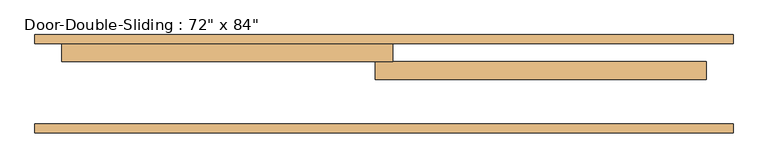
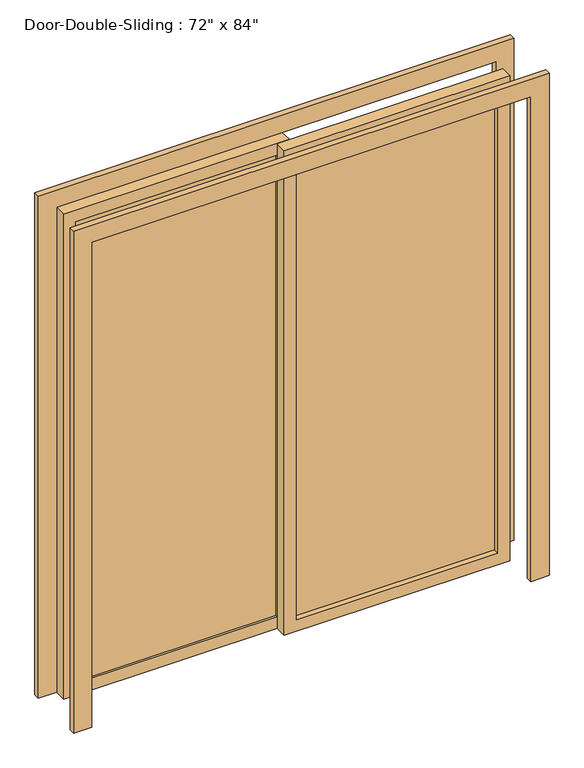
"""IFC4 building model written with IfcOpenShell, lengths in millimetres: door geometry."""

from ifc_helpers import new_model, si_unit, frame, origin, place, context, project, spatial, polyline, outline, extrude, source, transform, mapped, element, save


def door_d4d75d1e(model_context):
    return source(origin(), model_context, "Body", "SweptSolid", [
        extrude(outline(polyline([(0.0, 990.6), (2209.8, 990.6), (2209.8, -990.6), (0.0, -990.6), (0.0, -914.4), (2133.6, -914.4), (2133.6, 914.4), (0.0, 914.4), (0.0, 990.6)])), frame((0.0, 241.3, 0.0), z_axis=(0.0, 1.0, 0.0), x_axis=(0.0, 0.0, 1.0)), (0.0, 0.0, 1.0), 25.4),
        extrude(outline(polyline([(0.0, -990.6), (0.0, -914.4), (2133.6, -914.4), (2133.6, 914.4), (0.0, 914.4), (0.0, 990.6), (2209.8, 990.6), (2209.8, -990.6), (0.0, -990.6)])), frame((0.0, -12.7, 0.0), z_axis=(0.0, 1.0, 0.0), x_axis=(0.0, 0.0, 1.0)), (0.0, 0.0, 1.0), 25.4),
        extrude(outline(polyline([(2133.6, 25.4), (2133.6, -914.4), (0.0, -914.4), (0.0, 25.4), (2133.6, 25.4)]), holes=[polyline([(2082.8, -25.4), (50.8, -25.4), (50.8, -863.6), (2082.8, -863.6), (2082.8, -25.4)])]), frame((0.0, 190.5, 0.0), z_axis=(0.0, 1.0, 0.0), x_axis=(0.0, 0.0, 1.0)), (0.0, 0.0, 1.0), 50.8),
        extrude(outline(polyline([(2133.6, -25.4), (0.0, -25.4), (0.0, 914.4), (2133.6, 914.4), (2133.6, -25.4)]), holes=[polyline([(2082.8, 25.4), (2082.8, 863.6), (50.8, 863.6), (50.8, 25.4), (2082.8, 25.4)])]), frame((0.0, 139.7, 0.0), z_axis=(0.0, 1.0, 0.0), x_axis=(0.0, 0.0, 1.0)), (0.0, 0.0, 1.0), 50.8),
        extrude(outline(polyline([(-25.4, 200.025), (-863.6, 200.025), (-863.6, 206.375), (-25.4, 206.375), (-25.4, 200.025)])), frame((0.0, 0.0, 50.8), z_axis=(0.0, 0.0, 1.0), x_axis=(1.0, 0.0, 0.0)), (0.0, 0.0, 1.0), 2032.0),
        extrude(outline(polyline([(25.4, 168.275), (863.6, 168.275), (863.6, 161.925), (25.4, 161.925), (25.4, 168.275)])), frame((0.0, 0.0, 50.8), z_axis=(0.0, 0.0, 1.0), x_axis=(1.0, 0.0, 0.0)), (0.0, 0.0, 1.0), 2032.0),
    ])


if __name__ == "__main__":
    model = new_model("IFC4")
    model_context = context("Model", 3, world=origin())
    ifc_project = project(units=[si_unit("LENGTHUNIT", "METRE", prefix="MILLI")], contexts=[model_context])
    site = spatial("IfcSite", under=ifc_project)
    building = spatial("IfcBuilding", under=site)
    placement = place(None, origin())
    door_shape = door_d4d75d1e(model_context)
    element("IfcDoor", 1, ObjectType="Door-Double-Sliding : 72\" x 84\"", at=placement, inside=building, context=model_context, shape_type="MappedRepresentation", body=[
        mapped(door_shape, transform((0.0, 0.0, 0.0), x_axis=(1.0, 0.0, 0.0), y_axis=(0.0, 1.0, 0.0), z_axis=(0.0, 0.0, 1.0))),
    ])
    save(model, "model.ifc")

# Revit data of these elements
# Type "Door-Double-Sliding : 72\" x 84\""
#   Type Mark = "8"
#   Construction Type Id = "opn-d45"
#   Assembly Code = "C1020"
#   Analytic Construction = "Wood frame, double glass door "
#   Thickness = 0' - 2"
#   Thermal Resistance (R) = 1.8150 (h·ft²·°F)/BTU
#   Heat Transfer Coefficient (U) = 0.5510 BTU/(h·ft²·°F)
#   Height = 7' - 0"
#   Rail Width = 0' - 2"
#   Stiles = 0' - 2"
#   Trim Projection Ext = 0' - 1"
#   Trim Projection Int = 0' - 1"
#   Trim Width = 0' - 3"
#   Width = 6' - 0"
#   Define Thermal Properties by = 1
#   Glazing = Glass
#   Panel Material = Wood - Birch - Solid Stained Light Low Gloss
#   Trim Material = Paint - Sienna
#   Visual Light Transmittance = 0
#   Solar Heat Gain Coefficient = 0
#   Function = (empty or 0)
#   Wall Closure = (empty or 0)
# Element 1 (IfcDoor, "Door-Double-Sliding : 72\" x 84\"")
#   Materials on its faces: "Paint - Sienna", "Wood - Birch - Solid Stained Light Low Gloss", "Glass"
# Materials
#   "Glass": class "Glass", colour RGB 0 128 192, transparency 0.75, Description = "Soda Lime Glass", Cost = 0
#   "Wood - Birch - Solid Stained Light Low Gloss": class "Wood", colour RGB 210 159 95, transparency 0, Cost = 0
#   "Paint - Sienna": colour RGB 118 70 51, transparency 0, Cost = 0
